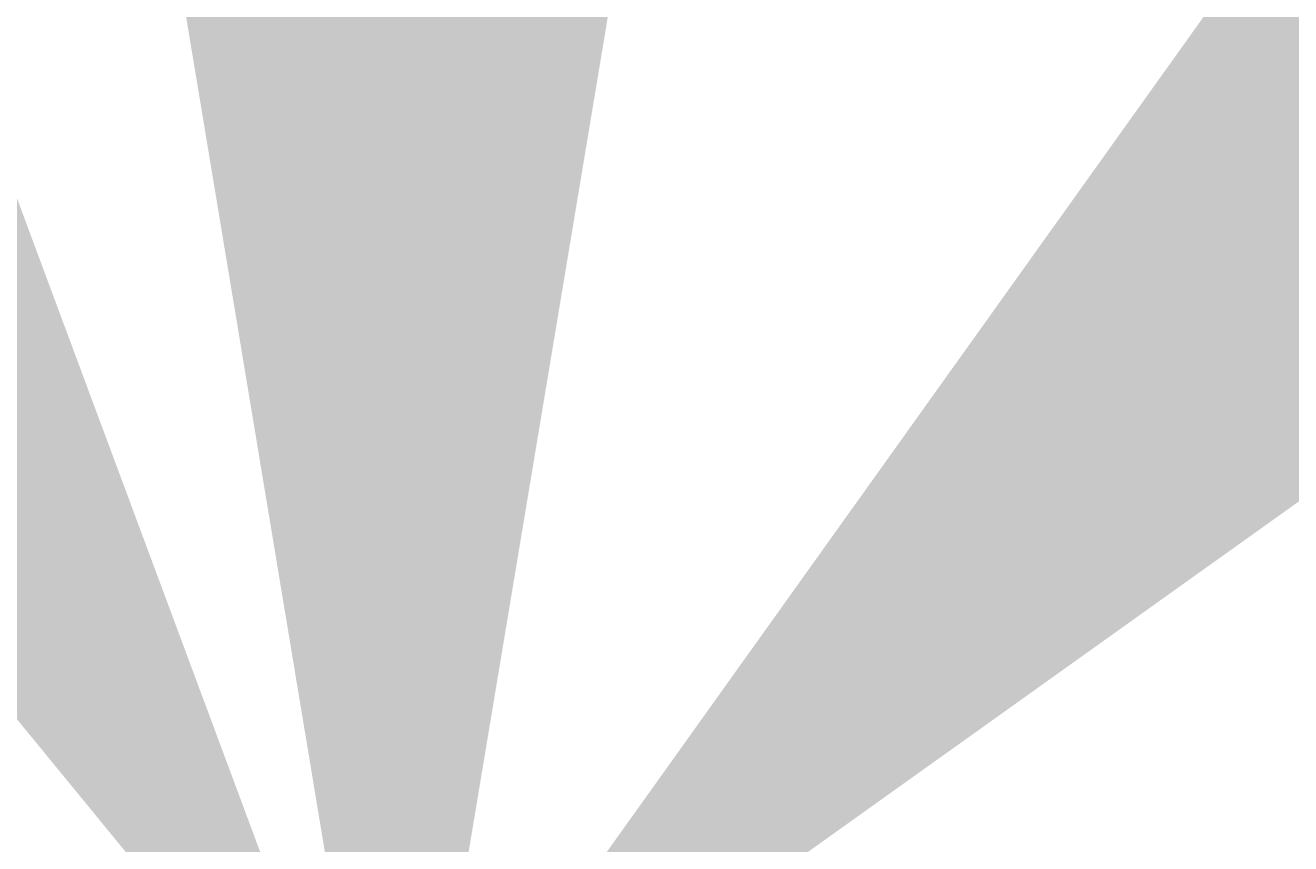
# Model space of a CAD drawing. Units: millimetres. Extents: x -22994 to 29398, y -19990 to 20176.
# Tile 132 of 135: x -2139 to 5745, y 2002 to 7102. Entities that reach past the tile are written whole.
import ezdxf

# ---------------------------------------------------------------- set-up
doc = ezdxf.new("R2010")
doc.units = ezdxf.units.MM
doc.header["$MEASUREMENT"] = 0
doc.layers.add('M-DIMS', color=2, linetype='Continuous', lineweight=18)
doc.styles.get("Standard").update_dxf_attribs({"font": 'arial.ttf'})
doc.dimstyles.get("Standard").update_dxf_attribs({"dimtxt": 0.18, "dimasz": 10000, "dimexe": 0.18, "dimexo": 0.0625, "dimgap": 0.09, "dimtad": 0, "dimtih": 1, "dimtoh": 1, "dimdec": 0, "dimzin": 0, "dimdsep": 46, "dimtxsty": 'Standard', "dimcen": 0.09, "dimadec": 0, "dimazin": 0, "dimtfac": 1, "dimtdec": 0, "dimtofl": 0, "dimtmove": 0, "dimatfit": 3, "dimfxl": 1, "dimtolj": 1, "dimtzin": 0, "dimlwd": 30, "dimarcsym": 0})

# ---------------------------------------------------------------- blocks, each defined once
blk = doc.blocks.new('*D9')
at = {"layer": 'Defpoints', "color": 0, "transparency": 16777216}
for p in [(187.3, 176.4), (306.2, 176.4), (290.9, 10.3)]:
    blk.add_point(p, dxfattribs=at)
at = {"layer": 'M-DIMS', "color": 0, "lineweight": 30, "transparency": 16777216}
for p, q in [((306.2, 10176.4), (306.2, 20176.4)), ((306.2, -9989.7), (306.2, -19989.7))]:
    blk.add_line(p, q, dxfattribs=at)
at = {"layer": 'M-DIMS', "color": 0, "lineweight": -2, "transparency": 16777216}
for p, q in [((187.3, 176.4), (306.4, 176.4)), ((290.9, 10.3), (306.4, 10.3))]:
    blk.add_line(p, q, dxfattribs=at)
at = {"layer": 'M-DIMS', "color": 0, "transparency": 16777216}
for points in [[(-1360.5, 10176.4), (1972.9, 10176.4), (306.2, 176.4)], [(-1360.5, -9989.7), (1972.9, -9989.7), (306.2, 10.3)]]:
    blk.add_solid(points, dxfattribs=at)
at = {"layer": 'M-DIMS', "color": 0, "transparency": 16777216, "insert": (306.2, 93.3), "char_height": 0.18, "attachment_point": 5}
blk.add_mtext('\\A1;166.1', dxfattribs=at)
blk = doc.blocks.new('*D15')
at = {"layer": 'Defpoints', "color": 0, "transparency": 16777216}
for p in [(173.3, 154.8), (173.3, 136.1), (306.2, 136.1)]:
    blk.add_point(p, dxfattribs=at)
at = {"layer": 'M-DIMS', "color": 0, "lineweight": 30, "transparency": 16777216}
for p, q in [((306.2, 10154.8), (306.2, 20154.8)), ((306.2, -9863.9), (306.2, -19863.9))]:
    blk.add_line(p, q, dxfattribs=at)
at = {"layer": 'M-DIMS', "color": 0, "lineweight": -2, "transparency": 16777216}
for p, q in [((173.4, 154.8), (306.4, 154.8)), ((173.4, 136.1), (306.4, 136.1))]:
    blk.add_line(p, q, dxfattribs=at)
at = {"layer": 'M-DIMS', "color": 0, "transparency": 16777216}
for points in [[(-1360.5, 10154.8), (1972.9, 10154.8), (306.2, 154.8)], [(-1360.5, -9863.9), (1972.9, -9863.9), (306.2, 136.1)]]:
    blk.add_solid(points, dxfattribs=at)
at = {"layer": 'M-DIMS', "color": 0, "transparency": 16777216, "insert": (306.2, 145.4), "char_height": 0.18, "attachment_point": 5}
blk.add_mtext('\\A1;18.717', dxfattribs=at)
blk = doc.blocks.new('*D28')
at = {"layer": 'Defpoints', "color": 0, "transparency": 16777216}
for p in [(188.1, 48), (188.1, 31), (306.2, 48)]:
    blk.add_point(p, dxfattribs=at)
at = {"layer": 'M-DIMS', "color": 0, "lineweight": 30, "transparency": 16777216}
for p, q in [((306.2, 10048), (306.2, 20048)), ((306.2, -9969), (306.2, -19969))]:
    blk.add_line(p, q, dxfattribs=at)
at = {"layer": 'M-DIMS', "color": 0, "lineweight": -2, "transparency": 16777216}
for p, q in [((188.2, 48), (306.4, 48)), ((188.2, 31), (306.4, 31))]:
    blk.add_line(p, q, dxfattribs=at)
at = {"layer": 'M-DIMS', "color": 0, "transparency": 16777216}
for points in [[(-1360.5, 10048), (1972.9, 10048), (306.2, 48)], [(-1360.5, -9969), (1972.9, -9969), (306.2, 31)]]:
    blk.add_solid(points, dxfattribs=at)
at = {"layer": 'M-DIMS', "color": 0, "transparency": 16777216, "insert": (306.2, 39.5), "char_height": 0.18, "attachment_point": 5}
blk.add_mtext('\\A1;17.045', dxfattribs=at)
blk = doc.blocks.new('*D34')
at = {"layer": 'Defpoints', "color": 0, "transparency": 16777216}
for p in [(176.8, 121.1), (178.6, 122.9)]:
    blk.add_point(p, dxfattribs=at)
at = {"layer": 'M-DIMS', "color": 0, "lineweight": 30, "transparency": 16777216}
for p, q in [((14322.4, 14263.3), (7250.5, 7193.1)), ((24322.4, 14263.3), (14322.4, 14263.3))]:
    blk.add_line(p, q, dxfattribs=at)
at = {"layer": 'M-DIMS', "color": 0, "lineweight": -2, "transparency": 16777216}
for p, q in [((176.7, 121.1), (176.9, 121.1)), ((176.8, 121), (176.8, 121.2))]:
    blk.add_line(p, q, dxfattribs=at)
at = {"layer": 'M-DIMS', "color": 0, "transparency": 16777216}
blk.add_solid([(6072.1, 8371.8), (8428.9, 6014.4), (178.6, 122.9)], dxfattribs=at)
at = {"layer": 'M-DIMS', "color": 0, "transparency": 16777216, "insert": (24323, 14263.3), "char_height": 0.18, "attachment_point": 5}
blk.add_mtext('\\A1;6X R2.5', dxfattribs=at)
blk = doc.blocks.new('*D35')
at = {"layer": 'Defpoints', "color": 0, "transparency": 16777216}
for p in [(21.1, 77.4), (21.8, 76.1)]:
    blk.add_point(p, dxfattribs=at)
at = {"layer": 'M-DIMS', "color": 0, "lineweight": 30, "transparency": 16777216}
for p, q in [((-19938, 17421.4), (-9938, 17421.4)), ((-9938, 17421.4), (-4958.5, 8749.4))]:
    blk.add_line(p, q, dxfattribs=at)
at = {"layer": 'M-DIMS', "color": 0, "lineweight": -2, "transparency": 16777216}
for p, q in [((21.8, 76), (21.8, 76.2)), ((21.8, 76.1), (21.9, 76.1))]:
    blk.add_line(p, q, dxfattribs=at)
at = {"layer": 'M-DIMS', "color": 0, "transparency": 16777216}
blk.add_solid([(-3513.1, 9579.3), (-6403.8, 7919.5), (21.1, 77.4)], dxfattribs=at)
at = {"layer": 'M-DIMS', "color": 0, "transparency": 16777216, "insert": (-19938.4, 17421.4), "char_height": 0.18, "attachment_point": 5}
blk.add_mtext('\\A1;R1.5', dxfattribs=at)
blk = doc.blocks.new('*D36')
at = {"layer": 'Defpoints', "color": 0, "transparency": 16777216}
for p in [(46.4, 31.3), (46.4, 26.6)]:
    blk.add_point(p, dxfattribs=at)
at = {"layer": 'M-DIMS', "color": 0, "lineweight": 30, "transparency": 16777216}
for p, q in [((57.1, 20031.3), (51.8, 10031.3)), ((10057.1, 20031.3), (57.1, 20031.3))]:
    blk.add_line(p, q, dxfattribs=at)
at = {"layer": 'M-DIMS', "color": 0, "lineweight": -2, "transparency": 16777216}
for p, q in [((46.3, 28.9), (46.5, 28.9)), ((46.4, 28.9), (46.4, 29))]:
    blk.add_line(p, q, dxfattribs=at)
at = {"layer": 'M-DIMS', "color": 0, "transparency": 16777216}
blk.add_solid([(-1614.9, 10032.2), (1718.4, 10030.4), (46.4, 31.3)], dxfattribs=at)
at = {"layer": 'M-DIMS', "color": 0, "transparency": 16777216, "insert": (10057.6, 20031.3), "char_height": 0.18, "attachment_point": 5}
blk.add_mtext('\\A1;∅4.71', dxfattribs=at)

msp = doc.modelspace()

# ---------------------------------------------------------------- dimensions: what is measured, and where the dimension line sits
at = {"layer": 'M-DIMS'}
for base, p1, p2, override, picture, middle in [((306.202, 176.3662), (290.852, 10.2713), (187.2647, 176.3662), {"dimdec": 1, "dimlfac": 1, "dimrnd": 0, "dimzin": 0, "dimdsep": 46, "dimlunit": 2}, '*D9', (306.202, 93.3187)), ((306.202, 136.0713), (173.3459, 154.788), (173.3459, 136.0713), {"dimdec": 3, "dimlfac": 1, "dimrnd": 0, "dimzin": 0, "dimdsep": 46, "dimlunit": 2}, '*D15', (306.202, 145.4297)), ((306.202, 48.0349), (188.1175, 30.9895), (188.1175, 48.0349), {"dimdec": 3, "dimlfac": 1, "dimrnd": 0, "dimzin": 0, "dimdsep": 46, "dimlunit": 2}, '*D28', (306.202, 39.5122))]:
    dim = msp.add_linear_dim(base=base, p1=p1, p2=p2, angle=90, dimstyle='Standard', override=override, dxfattribs=at)
    dim.commit()
    dim.dimension.update_dxf_attribs({"geometry": picture, "text_midpoint": middle})
dim = msp.add_diameter_dim_2p(p1=(46.3875, 26.5934), p2=(46.39, 31.3035), dimstyle='Standard', override={"dimdec": 2, "dimlfac": 1, "dimrnd": 0, "dimzin": 0, "dimdsep": 46, "dimlunit": 2}, dxfattribs=at)
dim.commit()
dim.dimension.update_dxf_attribs({"geometry": '*D36', "text_midpoint": (10057.5542, 20031.3006), "dimtype": 163})
dim = msp.add_radius_dim(center=(21.8402, 76.0922), mpoint=(21.0933, 77.393), dimstyle='Standard', override={"dimdec": 1, "dimlfac": 1, "dimrnd": 0, "dimzin": 0, "dimdsep": 46, "dimlunit": 2}, dxfattribs=at)
dim.commit()
dim.dimension.update_dxf_attribs({"geometry": '*D35', "text_midpoint": (-19938.3541, 17421.4466)})
dim = msp.add_radius_dim(center=(176.8123, 121.1277), mpoint=(178.5802, 122.8952), text='6X <>', dimstyle='Standard', override={"dimdec": 1, "dimlfac": 1, "dimrnd": 0, "dimzin": 0, "dimdsep": 46, "dimlunit": 2}, dxfattribs=at)
dim.commit()
dim.dimension.update_dxf_attribs({"geometry": '*D34', "text_midpoint": (24322.9703, 14263.3108)})

doc.saveas('drawing.dxf')
